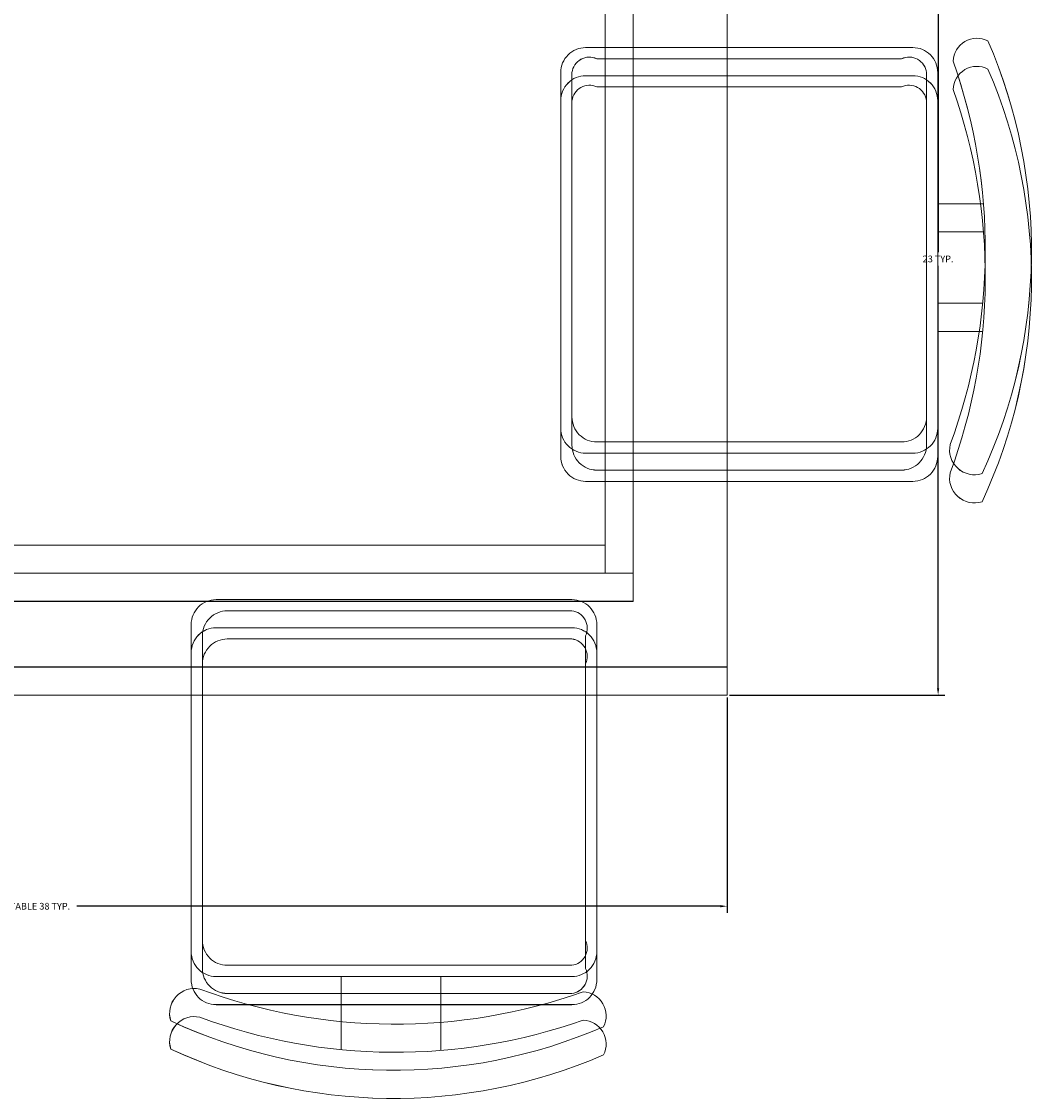
# Model space of a CAD drawing. Units: inches. Extents: x 1885 to 2748, y 783 to 2421.
# Tile 25 of 117: x 2367 to 2395, y 1245 to 1274. Entities that reach past the tile are written whole.
import ezdxf

# ---------------------------------------------------------------- set-up
doc = ezdxf.new("R2010")
doc.units = ezdxf.units.IN
doc.layers.add('A-ANNO-DIMS', color=2, linetype='Continuous', lineweight=18)
doc.layers.add('A-FURN', color=8, linetype='Continuous', lineweight=13)
doc.styles.get("Standard").update_dxf_attribs({"font": 'arial.ttf'})
doc.dimstyles.get("Standard").update_dxf_attribs({"dimtxt": 0.18, "dimasz": 0.18, "dimexe": 0.18, "dimexo": 0.0625, "dimgap": 0.09, "dimtad": 0, "dimtih": 1, "dimtoh": 1, "dimdec": 4, "dimzin": 0, "dimdsep": 46, "dimtxsty": 'Standard', "dimcen": 0.09, "dimadec": 0, "dimazin": 0, "dimtfac": 1, "dimtdec": 4, "dimtofl": 0, "dimtmove": 0, "dimatfit": 3, "dimfxl": 1, "dimtolj": 1, "dimtzin": 0, "dimarcsym": 0})

# ---------------------------------------------------------------- blocks, each defined once
blk = doc.blocks.new('TABLE-DINING-RECT')
for points in [[(-0.004, 23.421), (37.776, 23.421), (37.776, 0.754), (-0.004, 0.754)], [(-0.004, 23.421), (37.776, 23.421), (37.776, 0.753), (-0.004, 0.753)], [(-0.004, 22.666), (37.776, 22.666), (37.776, -0.002), (-0.004, -0.002)], [(-0.004, 22.665), (37.776, 22.665), (37.776, -0.002), (-0.004, -0.002)], [(2.515, 20.903), (35.257, 20.903), (35.257, 3.272), (2.515, 3.272)], [(2.515, 20.902), (35.257, 20.902), (35.257, 3.272), (2.515, 3.272)], [(2.515, 20.147), (35.257, 20.147), (35.257, 2.517), (2.515, 2.517)], [(2.515, 20.147), (35.257, 20.147), (35.257, 2.516), (2.515, 2.516)], [(3.27, 20.147), (34.501, 20.147), (34.501, 4.028), (3.27, 4.028)], [(3.27, 20.147), (34.501, 20.147), (34.501, 4.027), (3.27, 4.027)], [(3.27, 19.391), (34.501, 19.391), (34.501, 3.272), (3.27, 3.272)], [(3.27, 19.391), (34.501, 19.391), (34.501, 3.272), (3.27, 3.272)]]:
    blk.add_lwpolyline(points, close=True)
blk = doc.blocks.new('*D35')
at = {"layer": 'A-ANNO-DIMS', "color": 0, "lineweight": -2, "transparency": 16777216}
for p, q in [((2348.636, 1256.205), (2348.636, 1250.421)), ((2386.416, 1256.205), (2386.416, 1250.421)), ((2348.816, 1250.601), (2366.094, 1250.601)), ((2386.236, 1250.601), (2368.958, 1250.601))]:
    blk.add_line(p, q, dxfattribs=at)
at = {"layer": 'A-ANNO-DIMS', "color": 0, "transparency": 16777216}
for points in [[(2348.816, 1250.631), (2348.816, 1250.571), (2348.636, 1250.601)], [(2386.236, 1250.631), (2386.236, 1250.571), (2386.416, 1250.601)]]:
    blk.add_solid(points, dxfattribs=at)
at = {"layer": 'Defpoints', "color": 0, "transparency": 16777216}
for p in [(2348.636, 1256.268), (2386.416, 1256.268), (2386.416, 1250.601)]:
    blk.add_point(p, dxfattribs=at)
at = {"layer": 'A-ANNO-DIMS', "color": 0, "transparency": 16777216, "insert": (2367.526, 1250.601), "char_height": 0.18, "attachment_point": 5}
blk.add_mtext('\\A1;DINING TABLE 38 TYP.', dxfattribs=at)
blk = doc.blocks.new('*D36')
at = {"layer": 'A-ANNO-DIMS', "color": 0, "lineweight": -2, "transparency": 16777216}
for p, q in [((2386.478, 1279.691), (2392.263, 1279.691)), ((2392.083, 1279.511), (2392.083, 1268.161)), ((2392.083, 1256.448), (2392.083, 1267.797)), ((2386.478, 1256.268), (2392.263, 1256.268))]:
    blk.add_line(p, q, dxfattribs=at)
at = {"layer": 'A-ANNO-DIMS', "color": 0, "transparency": 16777216}
for points in [[(2392.053, 1279.511), (2392.113, 1279.511), (2392.083, 1279.691)], [(2392.053, 1256.448), (2392.113, 1256.448), (2392.083, 1256.268)]]:
    blk.add_solid(points, dxfattribs=at)
at = {"layer": 'Defpoints', "color": 0, "transparency": 16777216}
for p in [(2386.416, 1279.691), (2392.083, 1279.691), (2386.416, 1256.268)]:
    blk.add_point(p, dxfattribs=at)
at = {"layer": 'A-ANNO-DIMS', "color": 0, "transparency": 16777216, "insert": (2392.083, 1267.979), "char_height": 0.18, "attachment_point": 5}
blk.add_mtext('\\A1;23 TYP.', dxfattribs=at)

msp = doc.modelspace()

# ---------------------------------------------------------------- linework, layer by layer
at = {"layer": 'A-FURN'}
for points in [[(2392.485, 1273.286, -0.175809), (2392.407, 1262.996, 0.578392), (2393.264, 1262.216, 0.214524), (2393.42, 1273.832, 0.552014), (2392.485, 1273.286, -0.065079)], [(2392.485, 1273.285, -0.175809), (2392.407, 1262.995, 0.578392), (2393.264, 1262.216, 0.214524), (2393.42, 1273.831, 0.552014), (2392.485, 1273.285, -0.065079)], [(2392.072, 1272.985, 0.414214), (2391.404, 1273.654), (2382.62, 1273.654, 0.414214), (2381.952, 1272.985), (2381.952, 1263.432, 0.414214), (2382.62, 1262.764), (2391.404, 1262.764, 0.414214), (2392.072, 1263.432), (2392.072, 1272.985)], [(2392.072, 1272.985, 0.414214), (2391.404, 1273.653), (2382.62, 1273.653, 0.414214), (2381.952, 1272.985), (2381.952, 1263.432, 0.414214), (2382.62, 1262.764), (2391.404, 1262.764, 0.414214), (2392.072, 1263.432), (2392.072, 1272.985)], [(2392.485, 1272.53, -0.175809), (2392.407, 1262.24, 0.578392), (2393.264, 1261.461, 0.214524), (2393.42, 1273.076, 0.552014), (2392.485, 1272.53, -0.065079)], [(2392.485, 1272.53, -0.175809), (2392.407, 1262.24, 0.578392), (2393.264, 1261.46, 0.214524), (2393.42, 1273.076, 0.552014), (2392.485, 1272.53, -0.065079)], [(2392.072, 1272.23, 0.414214), (2391.404, 1272.898), (2382.62, 1272.898, 0.414214), (2381.952, 1272.23), (2381.952, 1262.677, 0.414214), (2382.62, 1262.008), (2391.404, 1262.008, 0.414214), (2392.072, 1262.677), (2392.072, 1272.23)], [(2392.072, 1272.229, 0.414214), (2391.404, 1272.898), (2382.62, 1272.898, 0.414214), (2381.952, 1272.229), (2381.952, 1262.676, 0.414214), (2382.62, 1262.008), (2391.404, 1262.008, 0.414214), (2392.072, 1262.676), (2392.072, 1272.229)], [(2392.072, 1266.788), (2393.28, 1266.788, -0.064759)], [(2392.072, 1266.787), (2393.28, 1266.787, -0.064759)], [(2392.072, 1266.032), (2393.28, 1266.032, -0.064759)], [(2392.072, 1266.032), (2393.28, 1266.032, -0.064759)], [(2382.252, 1248.713, 0.414214), (2382.92, 1249.381), (2382.92, 1258.165, 0.414214), (2382.252, 1258.833), (2372.699, 1258.833, 0.414214), (2372.03, 1258.165), (2372.03, 1249.381, 0.414214), (2372.699, 1248.713), (2382.252, 1248.713)], [(2382.252, 1248.713, 0.414214), (2382.92, 1249.381), (2382.92, 1258.165, 0.414214), (2382.252, 1258.833), (2372.699, 1258.833, 0.414214), (2372.03, 1258.165), (2372.03, 1249.381, 0.414214), (2372.699, 1248.713), (2382.252, 1248.713)], [(2382.252, 1247.958, 0.414214), (2382.92, 1248.626), (2382.92, 1257.41, 0.414214), (2382.252, 1258.078), (2372.699, 1258.078, 0.414214), (2372.03, 1257.41), (2372.03, 1248.626, 0.414214), (2372.699, 1247.958), (2382.252, 1247.958)], [(2382.252, 1247.957, 0.414214), (2382.92, 1248.625), (2382.92, 1257.409, 0.414214), (2382.252, 1258.077), (2372.699, 1258.077, 0.414214), (2372.03, 1257.409), (2372.03, 1248.625, 0.414214), (2372.699, 1247.957), (2382.252, 1247.957)], [(2376.054, 1248.713), (2376.054, 1247.505, -0.064759)], [(2376.054, 1248.713), (2376.054, 1247.505, -0.064759)], [(2382.552, 1248.3, -0.175809), (2372.262, 1248.378, 0.578392), (2371.482, 1247.521, 0.214524), (2383.098, 1247.365, 0.552014), (2382.552, 1248.3, -0.065079)], [(2382.552, 1248.3, -0.175809), (2372.262, 1248.378, 0.578392), (2371.483, 1247.52, 0.214524), (2383.098, 1247.365, 0.552014), (2382.552, 1248.3, -0.065079)], [(2376.054, 1247.958), (2376.054, 1246.749, -0.064759)], [(2376.054, 1247.957), (2376.054, 1246.749, -0.064759)], [(2382.552, 1247.545, -0.175809), (2372.262, 1247.622, 0.578392), (2371.482, 1246.765, 0.214524), (2383.098, 1246.609, 0.552014), (2382.552, 1247.545, -0.065079)], [(2382.552, 1247.544, -0.175809), (2372.262, 1247.622, 0.578392), (2371.483, 1246.765, 0.214524), (2383.098, 1246.609, 0.552014), (2382.552, 1247.544, -0.065079)]]:
    msp.add_lwpolyline(points, format="xyb", dxfattribs=at)
for points in [[(2391.771, 1272.981), (2391.771, 1263.733, -0.414214), (2391.102, 1263.065), (2382.921, 1263.065, -0.414214), (2382.253, 1263.733), (2382.253, 1272.981, -0.512069), (2382.921, 1273.353), (2391.102, 1273.353, -0.512069)], [(2391.771, 1272.981), (2391.771, 1263.733, -0.414214), (2391.102, 1263.065), (2382.921, 1263.065, -0.414214), (2382.253, 1263.733), (2382.253, 1272.981, -0.512069), (2382.921, 1273.352), (2391.102, 1273.352, -0.512069)], [(2391.771, 1272.226), (2391.771, 1262.978, -0.414214), (2391.102, 1262.31), (2382.921, 1262.31, -0.414214), (2382.253, 1262.978), (2382.253, 1272.226, -0.512069), (2382.921, 1272.597), (2391.102, 1272.597, -0.512069)], [(2391.771, 1272.225), (2391.771, 1262.978, -0.414214), (2391.102, 1262.309), (2382.921, 1262.309, -0.414214), (2382.253, 1262.978), (2382.253, 1272.225, -0.512069), (2382.921, 1272.597), (2391.102, 1272.597, -0.512069)], [(2382.247, 1249.014), (2373, 1249.014, -0.414214), (2372.331, 1249.683), (2372.331, 1257.864, -0.414214), (2373, 1258.532), (2382.247, 1258.532, -0.512069), (2382.619, 1257.864), (2382.619, 1249.683, -0.512069)], [(2382.247, 1249.014), (2373, 1249.014, -0.414214), (2372.331, 1249.682), (2372.331, 1257.864, -0.414214), (2373, 1258.532), (2382.247, 1258.532, -0.512069), (2382.619, 1257.864), (2382.619, 1249.682, -0.512069)], [(2382.247, 1248.259), (2373, 1248.259, -0.414214), (2372.331, 1248.927), (2372.331, 1257.108, -0.414214), (2373, 1257.777), (2382.247, 1257.777, -0.512069), (2382.619, 1257.108), (2382.619, 1248.927, -0.512069)], [(2382.247, 1248.258), (2373, 1248.258, -0.414214), (2372.331, 1248.927), (2372.331, 1257.108, -0.414214), (2373, 1257.776), (2382.247, 1257.776, -0.512069), (2382.619, 1257.108), (2382.619, 1248.927, -0.512069)]]:
    msp.add_lwpolyline(points, format="xyb", close=True, dxfattribs=at)
for points in [[(2393.302, 1269.462), (2392.072, 1269.462)], [(2393.302, 1269.461), (2392.072, 1269.461)], [(2393.302, 1268.706), (2392.072, 1268.706)], [(2393.302, 1268.706), (2392.072, 1268.706)], [(2378.728, 1247.483), (2378.728, 1248.713)], [(2378.728, 1247.483), (2378.728, 1248.713)], [(2378.728, 1246.727), (2378.728, 1247.958)], [(2378.728, 1246.727), (2378.728, 1247.957)]]:
    msp.add_lwpolyline(points, dxfattribs=at)

# ---------------------------------------------------------------- block references
msp.add_blockref('TABLE-DINING-RECT', (2348.64, 1256.27), dxfattribs=at)

# ---------------------------------------------------------------- dimensions: what is measured, and where the dimension line sits
at = {"layer": 'A-ANNO-DIMS'}
dim = msp.add_linear_dim(base=(2392.083, 1279.691), p1=(2386.416, 1256.268), p2=(2386.416, 1279.691), angle=90, text='<> TYP.', dimstyle='Standard', override={"dimdec": 0, "dimlfac": 1, "dimrnd": 0, "dimzin": 0, "dimdsep": 46, "dimlunit": 2}, dxfattribs=at)
dim.commit()
dim.dimension.update_dxf_attribs({"geometry": '*D36', "text_midpoint": (2392.083, 1267.979)})
dim = msp.add_linear_dim(base=(2386.416, 1250.601), p1=(2348.636, 1256.268), p2=(2386.416, 1256.268), text='DINING TABLE <> TYP.', dimstyle='Standard', override={"dimdec": 0, "dimlfac": 1, "dimrnd": 0, "dimzin": 0, "dimdsep": 46, "dimlunit": 2}, dxfattribs=at)
dim.commit()
dim.dimension.update_dxf_attribs({"geometry": '*D35', "text_midpoint": (2367.526, 1250.601)})

doc.saveas('drawing.dxf')
